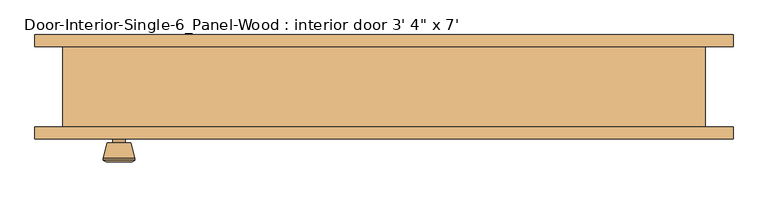
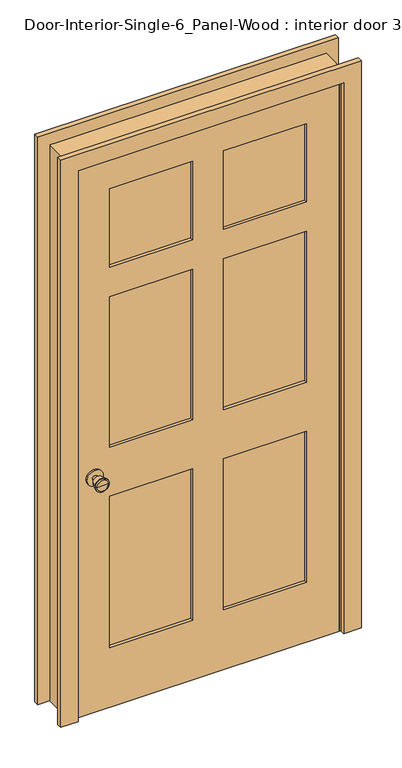
"""IFC4 building model written with IfcOpenShell, lengths in millimetres: door geometry."""

from ifc_helpers import new_model, si_unit, point, frame, frame_2d, origin, place, context, project, spatial, polyline, circle_curve, trimmed, segment, composite_curve, outline, extrude, faceted_brep, source, transform, mapped, element, save
from ifc_brep_helpers import plane_surface, cylinder_surface, revolved_surface, advanced_brep


def door_6a452240(model_context):
    return source(origin(), model_context, "Body", "SolidModel", [
        advanced_brep(
        [(-419.1, -19.4, 914.4), (-429.1, -19.4, 914.4), (-409.1, -19.4, 914.4), (-398.6241324, 29.6, 914.4), (-439.5758676, 29.6, 914.4), (-419.1, 29.6, 914.4), (-394.1, 27.7721319, 914.4), (-444.1, 27.7721319, 914.4), (-394.1, 24.3084537, 914.4), (-444.1, 24.3084537, 914.4), (-400.463764, -0.4, 914.4), (-437.736236, -0.4, 914.4), (-409.1, -0.4, 914.4), (-429.1, -0.4, 914.4)],
        [
            (0, 1),
            (1, 2, circle_curve(frame((-419.1, -19.4, 914.4), z_axis=(0.0, -1.0, 0.0), x_axis=(-1.0, 0.0, 0.0)), 10.0)),
            (2, 0),
            (2, 1, circle_curve(frame((-419.1, -19.4, 914.4), z_axis=(0.0, -1.0, 0.0), x_axis=(-1.0, 0.0, 0.0)), 10.0)),
            (3, 4, circle_curve(frame((-419.1, 29.6, 914.4), z_axis=(0.0, 1.0, 0.0), x_axis=(-1.0, 0.0, 0.0)), 20.4758676)),
            (4, 5),
            (5, 3),
            (4, 3, circle_curve(frame((-419.1, 29.6, 914.4), z_axis=(0.0, 1.0, 0.0), x_axis=(-1.0, 0.0, 0.0)), 20.4758676)),
            (6, 7, circle_curve(frame((-419.1, 27.7721319, 914.4), z_axis=(0.0, 1.0, 0.0), x_axis=(-1.0, 0.0, 0.0)), 25.0)),
            (7, 4),
            (3, 6),
            (7, 6, circle_curve(frame((-419.1, 27.7721319, 914.4), z_axis=(0.0, 1.0, 0.0), x_axis=(-1.0, 0.0, 0.0)), 25.0)),
            (8, 9, circle_curve(frame((-419.1, 24.3084537, 914.4), z_axis=(0.0, 1.0, 0.0), x_axis=(-1.0, 0.0, 0.0)), 25.0)),
            (9, 7),
            (6, 8),
            (9, 8, circle_curve(frame((-419.1, 24.3084537, 914.4), z_axis=(0.0, 1.0, 0.0), x_axis=(-1.0, 0.0, 0.0)), 25.0)),
            (10, 11, circle_curve(frame((-419.1, -0.4, 914.4), z_axis=(0.0, 1.0, 0.0), x_axis=(-1.0, 0.0, 0.0)), 18.636236)),
            (11, 9),
            (8, 10),
            (11, 10, circle_curve(frame((-419.1, -0.4, 914.4), z_axis=(0.0, 1.0, 0.0), x_axis=(-1.0, 0.0, 0.0)), 18.636236)),
            (12, 13, circle_curve(frame((-419.1, -0.4, 914.4), z_axis=(0.0, 1.0, 0.0), x_axis=(-1.0, 0.0, 0.0)), 10.0)),
            (13, 11),
            (10, 12),
            (13, 12, circle_curve(frame((-419.1, -0.4, 914.4), z_axis=(0.0, 1.0, 0.0), x_axis=(-1.0, 0.0, 0.0)), 10.0)),
            (1, 13),
            (12, 2),
        ],
        [
            plane_surface(frame((-419.1, -19.4, 914.4), z_axis=(0.0, -1.0, 0.0), x_axis=(-1.0, 0.0, 0.0))),
            plane_surface(frame((-419.1, 29.6, 914.4), z_axis=(0.0, 1.0, 0.0), x_axis=(-1.0, 0.0, 0.0))),
            revolved_surface(polyline([(-439.5758676, 29.6, 914.4), (-444.1, 27.7721319, 914.4)]), (-419.1, -19.4, 914.4), (0.0, -1.0, 0.0)),
            cylinder_surface(frame((-419.1, -19.4, 914.4), z_axis=(0.0, -1.0, 0.0), x_axis=(-1.0, 0.0, 0.0)), 25.0),
            revolved_surface(polyline([(-444.1, 24.3084537, 914.4), (-437.736236, -0.4, 914.4)]), (-419.1, -19.4, 914.4), (0.0, -1.0, 0.0)),
            plane_surface(frame((-419.1, -0.4, 914.4), z_axis=(0.0, -1.0, 0.0), x_axis=(-1.0, 0.0, 0.0))),
            cylinder_surface(frame((-419.1, -19.4, 914.4), z_axis=(0.0, -1.0, 0.0), x_axis=(-1.0, 0.0, 0.0)), 10.0),
        ],
        [
            (0, [[1, 2, 3]]),
            (0, [[-3, 4, -1]]),
            (1, [[5, 6, 7]]),
            (1, [[8, -7, -6]]),
            (2, [[9, 10, -5, 11]]),
            (2, [[12, -11, -8, -10]]),
            (3, [[13, 14, -9, 15]]),
            (3, [[16, -15, -12, -14]]),
            (4, [[17, 18, -13, 19]]),
            (4, [[20, -19, -16, -18]]),
            (5, [[21, 22, -17, 23]]),
            (5, [[24, -23, -20, -22]]),
            (6, [[-2, 25, -21, 26]]),
            (6, [[-4, -26, -24, -25]]),
        ],
    ),
        extrude(outline(composite_curve([segment(trimmed(circle_curve(frame_2d((914.4, -419.1)), 30.0), [point((914.4, -449.1))], [point((914.4, -389.1))], False, "CARTESIAN"), True, "CONTINUOUS"), segment(trimmed(circle_curve(frame_2d((914.4, -419.1)), 30.0), [point((914.4, -389.1))], [point((914.4, -449.1))], False, "CARTESIAN"), True, "CONTINUOUS")], self_intersect=False)), frame((0.0, -25.4, 0.0), z_axis=(0.0, 1.0, 0.0), x_axis=(0.0, 0.0, 1.0)), (0.0, 0.0, 1.0), 6.0),
        advanced_brep(
        [(-419.1, -66.325, 914.4), (-409.1, -66.325, 914.4), (-429.1, -66.325, 914.4), (-398.6241324, -115.325, 914.4), (-419.1, -115.325, 914.4), (-439.5758676, -115.325, 914.4), (-394.1, -113.4971319, 914.4), (-444.1, -113.4971319, 914.4), (-394.1, -110.0334537, 914.4), (-444.1, -110.0334537, 914.4), (-400.463764, -85.325, 914.4), (-437.736236, -85.325, 914.4), (-409.1, -85.325, 914.4), (-429.1, -85.325, 914.4)],
        [
            (0, 1),
            (1, 2, circle_curve(frame((-419.1, -66.325, 914.4), z_axis=(0.0, 1.0, 0.0), x_axis=(-1.0, 0.0, 0.0)), 10.0)),
            (2, 0),
            (2, 1, circle_curve(frame((-419.1, -66.325, 914.4), z_axis=(0.0, 1.0, 0.0), x_axis=(-1.0, 0.0, 0.0)), 10.0)),
            (3, 4),
            (4, 5),
            (5, 3, circle_curve(frame((-419.1, -115.325, 914.4), z_axis=(0.0, -1.0, 0.0), x_axis=(-1.0, 0.0, 0.0)), 20.4758676)),
            (3, 5, circle_curve(frame((-419.1, -115.325, 914.4), z_axis=(0.0, -1.0, 0.0), x_axis=(-1.0, 0.0, 0.0)), 20.4758676)),
            (6, 3),
            (5, 7),
            (7, 6, circle_curve(frame((-419.1, -113.4971319, 914.4), z_axis=(0.0, -1.0, 0.0), x_axis=(-1.0, 0.0, 0.0)), 25.0)),
            (6, 7, circle_curve(frame((-419.1, -113.4971319, 914.4), z_axis=(0.0, -1.0, 0.0), x_axis=(-1.0, 0.0, 0.0)), 25.0)),
            (8, 6),
            (7, 9),
            (9, 8, circle_curve(frame((-419.1, -110.0334537, 914.4), z_axis=(0.0, -1.0, 0.0), x_axis=(-1.0, 0.0, 0.0)), 25.0)),
            (8, 9, circle_curve(frame((-419.1, -110.0334537, 914.4), z_axis=(0.0, -1.0, 0.0), x_axis=(-1.0, 0.0, 0.0)), 25.0)),
            (10, 8),
            (9, 11),
            (11, 10, circle_curve(frame((-419.1, -85.325, 914.4), z_axis=(0.0, -1.0, 0.0), x_axis=(-1.0, 0.0, 0.0)), 18.636236)),
            (10, 11, circle_curve(frame((-419.1, -85.325, 914.4), z_axis=(0.0, -1.0, 0.0), x_axis=(-1.0, 0.0, 0.0)), 18.636236)),
            (12, 10),
            (11, 13),
            (13, 12, circle_curve(frame((-419.1, -85.325, 914.4), z_axis=(0.0, -1.0, 0.0), x_axis=(-1.0, 0.0, 0.0)), 10.0)),
            (12, 13, circle_curve(frame((-419.1, -85.325, 914.4), z_axis=(0.0, -1.0, 0.0), x_axis=(-1.0, 0.0, 0.0)), 10.0)),
            (1, 12),
            (13, 2),
        ],
        [
            plane_surface(frame((-419.1, -66.325, 914.4), z_axis=(0.0, 1.0, 0.0), x_axis=(-1.0, 0.0, 0.0))),
            plane_surface(frame((-419.1, -115.325, 914.4), z_axis=(0.0, -1.0, 0.0), x_axis=(-1.0, 0.0, 0.0))),
            revolved_surface(polyline([(-439.5758676, -115.325, 914.4), (-444.1, -113.4971319, 914.4)]), (-419.1, -66.325, 914.4), (0.0, 1.0, 0.0)),
            cylinder_surface(frame((-419.1, -66.325, 914.4), z_axis=(0.0, 1.0, 0.0), x_axis=(-1.0, 0.0, 0.0)), 25.0),
            revolved_surface(polyline([(-444.1, -110.0334537, 914.4), (-437.736236, -85.325, 914.4)]), (-419.1, -66.325, 914.4), (0.0, 1.0, 0.0)),
            plane_surface(frame((-419.1, -85.325, 914.4), z_axis=(0.0, 1.0, 0.0), x_axis=(-1.0, 0.0, 0.0))),
            cylinder_surface(frame((-419.1, -66.325, 914.4), z_axis=(0.0, 1.0, 0.0), x_axis=(-1.0, 0.0, 0.0)), 10.0),
        ],
        [
            (0, [[1, 2, 3]]),
            (0, [[-3, 4, -1]]),
            (1, [[5, 6, 7]]),
            (1, [[-6, -5, 8]]),
            (2, [[9, -7, 10, 11]]),
            (2, [[-10, -8, -9, 12]]),
            (3, [[13, -11, 14, 15]]),
            (3, [[-14, -12, -13, 16]]),
            (4, [[17, -15, 18, 19]]),
            (4, [[-18, -16, -17, 20]]),
            (5, [[21, -19, 22, 23]]),
            (5, [[-22, -20, -21, 24]]),
            (6, [[25, -23, 26, -2]]),
            (6, [[-26, -24, -25, -4]]),
        ],
    ),
        extrude(outline(composite_curve([segment(trimmed(circle_curve(frame_2d((914.4, -419.1)), 30.0), [point((914.4, -449.1))], [point((914.4, -389.1))], False, "CARTESIAN"), True, "CONTINUOUS"), segment(trimmed(circle_curve(frame_2d((914.4, -419.1)), 30.0), [point((914.4, -389.1))], [point((914.4, -449.1))], False, "CARTESIAN"), True, "CONTINUOUS")], self_intersect=False)), frame((0.0, -66.325, 0.0), z_axis=(0.0, 1.0, 0.0), x_axis=(0.0, 0.0, 1.0)), (0.0, 0.0, 1.0), 6.0),
        faceted_brep([(508.0, -60.325, 0.0), (482.6, -60.325, 0.0), (482.6, -25.4, 0.0), (469.9, -25.4, 0.0), (469.9, 9.525, 0.0), (482.6, 9.525, 0.0), (482.6, 66.675, 0.0), (508.0, 66.675, 0.0), (508.0, 66.675, 2159.0), (508.0, -60.325, 2159.0), (482.6, 66.675, 2133.6), (-482.6, 66.675, 2133.6), (-482.6, 66.675, 0.0), (-508.0, 66.675, 0.0), (-508.0, 66.675, 2159.0), (482.6, 9.525, 2133.6), (469.9, 9.525, 2120.9), (-469.9, 9.525, 2120.9), (-469.9, 9.525, 0.0), (-482.6, 9.525, 0.0), (-482.6, 9.525, 2133.6), (469.9, -25.4, 2120.9), (482.6, -25.4, 2133.6), (-482.6, -25.4, 2133.6), (-482.6, -25.4, 0.0), (-469.9, -25.4, 0.0), (-469.9, -25.4, 2120.9), (482.6, -60.325, 2133.6), (-508.0, -60.325, 2159.0), (-508.0, -60.325, 0.0), (-482.6, -60.325, 0.0), (-482.6, -60.325, 2133.6)], [[[0, 1, 2, 3, 4, 5, 6, 7]], [[7, 8, 9, 0]], [[6, 10, 11, 12, 13, 14, 8, 7]], [[5, 15, 10, 6]], [[4, 16, 17, 18, 19, 20, 15, 5]], [[3, 21, 16, 4]], [[2, 22, 23, 24, 25, 26, 21, 3]], [[1, 27, 22, 2]], [[0, 9, 28, 29, 30, 31, 27, 1]], [[8, 14, 28, 9]], [[15, 20, 11, 10]], [[21, 26, 17, 16]], [[27, 31, 23, 22]], [[29, 13, 12, 19, 18, 25, 24, 30]], [[14, 13, 29, 28]], [[20, 19, 12, 11]], [[26, 25, 18, 17]], [[31, 30, 24, 23]]]),
        extrude(outline(polyline([(2133.6, -482.6), (0.0, -482.6), (0.0, 482.6), (2133.6, 482.6), (2133.6, -482.6)]), holes=[polyline([(2014.5375, 57.15), (2014.5375, 361.95), (1709.7375, 361.95), (1709.7375, 57.15), (2014.5375, 57.15)]), polyline([(1595.4375, 361.95), (1009.65, 361.95), (1009.65, 57.15), (1595.4375, 57.15), (1595.4375, 361.95)]), polyline([(1009.65, -57.15), (1009.65, -361.95), (1595.4375, -361.95), (1595.4375, -57.15), (1009.65, -57.15)]), polyline([(1709.7375, -361.95), (2014.5375, -361.95), (2014.5375, -57.15), (1709.7375, -57.15), (1709.7375, -361.95)]), polyline([(819.15, 57.15), (819.15, 361.95), (231.775, 361.95), (231.775, 57.15), (819.15, 57.15)]), polyline([(231.775, -57.15), (231.775, -361.95), (819.15, -361.95), (819.15, -57.15), (231.775, -57.15)])]), frame((0.0, -60.325, 0.0), z_axis=(0.0, 1.0, 0.0), x_axis=(0.0, 0.0, 1.0)), (0.0, 0.0, 1.0), 34.925),
        extrude(outline(polyline([(361.95, -37.0416667), (361.95, -48.6833333), (57.15, -48.6833333), (57.15, -37.0416667), (361.95, -37.0416667)])), frame((0.0, 0.0, 1709.7375), z_axis=(0.0, 0.0, 1.0), x_axis=(1.0, 0.0, 0.0)), (0.0, 0.0, 1.0), 304.8),
        extrude(outline(polyline([(361.95, -37.0416667), (361.95, -48.6833333), (57.15, -48.6833333), (57.15, -37.0416667), (361.95, -37.0416667)])), frame((0.0, 0.0, 1009.65), z_axis=(0.0, 0.0, 1.0), x_axis=(1.0, 0.0, 0.0)), (0.0, 0.0, 1.0), 585.7875),
        extrude(outline(polyline([(-57.15, -37.0416667), (-57.15, -48.6833333), (-361.95, -48.6833333), (-361.95, -37.0416667), (-57.15, -37.0416667)])), frame((0.0, 0.0, 1009.65), z_axis=(0.0, 0.0, 1.0), x_axis=(1.0, 0.0, 0.0)), (0.0, 0.0, 1.0), 585.7875),
        extrude(outline(polyline([(-57.15, -37.0416667), (-57.15, -48.6833333), (-361.95, -48.6833333), (-361.95, -37.0416667), (-57.15, -37.0416667)])), frame((0.0, 0.0, 1709.7375), z_axis=(0.0, 0.0, 1.0), x_axis=(1.0, 0.0, 0.0)), (0.0, 0.0, 1.0), 304.8),
        extrude(outline(polyline([(361.95, -37.0416667), (361.95, -48.6833333), (57.15, -48.6833333), (57.15, -37.0416667), (361.95, -37.0416667)])), frame((0.0, 0.0, 231.775), z_axis=(0.0, 0.0, 1.0), x_axis=(1.0, 0.0, 0.0)), (0.0, 0.0, 1.0), 587.375),
        extrude(outline(polyline([(-57.15, -37.0416667), (-57.15, -48.6833333), (-361.95, -48.6833333), (-361.95, -37.0416667), (-57.15, -37.0416667)])), frame((0.0, 0.0, 231.775), z_axis=(0.0, 0.0, 1.0), x_axis=(1.0, 0.0, 0.0)), (0.0, 0.0, 1.0), 587.375),
        extrude(outline(polyline([(0.0, 552.45), (2203.45, 552.45), (2203.45, -552.45), (0.0, -552.45), (0.0, -488.95), (2139.95, -488.95), (2139.95, 488.95), (0.0, 488.95), (0.0, 552.45)])), frame((0.0, -79.375, 0.0), z_axis=(0.0, 1.0, 0.0), x_axis=(0.0, 0.0, 1.0)), (0.0, 0.0, 1.0), 19.05),
        extrude(outline(polyline([(0.0, 552.45), (2203.45, 552.45), (2203.45, -552.45), (0.0, -552.45), (0.0, -488.95), (2139.95, -488.95), (2139.95, 488.95), (0.0, 488.95), (0.0, 552.45)])), frame((0.0, 66.675, 0.0), z_axis=(0.0, 1.0, 0.0), x_axis=(0.0, 0.0, 1.0)), (0.0, 0.0, 1.0), 19.05),
    ])


if __name__ == "__main__":
    model = new_model("IFC4")
    model_context = context("Model", 3, world=origin())
    ifc_project = project(units=[si_unit("LENGTHUNIT", "METRE", prefix="MILLI")], contexts=[model_context])
    site = spatial("IfcSite", under=ifc_project)
    building = spatial("IfcBuilding", under=site)
    placement = place(None, origin())
    door_shape = door_6a452240(model_context)
    element("IfcDoor", 1, ObjectType="Door-Interior-Single-6_Panel-Wood : interior door 3' 4\" x 7'", at=placement, inside=building, context=model_context, shape_type="MappedRepresentation", body=[
        mapped(door_shape, transform((0.0, 0.0, 0.0), x_axis=(1.0, 0.0, 0.0), y_axis=(0.0, 1.0, 0.0), z_axis=(0.0, 0.0, 1.0))),
    ])
    save(model, "model.ifc")

# Revit data of these elements
# Type "Door-Interior-Single-6_Panel-Wood : interior door 3' 4\" x 7'"
#   Type Mark = "11"
#   Assembly Code = "C1020300"
#   Analytic Construction = "Wooden"
#   Top Rail = 0' - 4 11/16"
#   Top Panel = 1' - 0"
#   Thickness = 0' - 1 3/8"
#   Thermal Resistance (R) = 2.5876 (h·ft²·°F)/BTU
#   Swing Angle [instance default] = 90.00°
#   Stiles = 0' - 4 3/4"
#   Rough Width = 3' - 4"
#   Rough Height = 7' - 1"
#   Mullion = 0' - 4 1/2"
#   Lock Rail = 0' - 7 1/2"
#   Intermediate Rail = 0' - 4 1/2"
#   Height = 7' - 0"
#   Width = 3' - 2"
#   Heat Transfer Coefficient (U) = 0.3865 BTU/(h·ft²·°F)
#   Bottom Rail = 0' - 9 1/8"
#   Trim Material = Cherry
#   Panel Material = Cherry
#   Frame Material = Cherry
#   Door Handle Material = Aluminum
#   Visual Light Transmittance = 0
#   Solar Heat Gain Coefficient = 0
#   Wall Closure = (empty or 0)
#   Function = (empty or 0)
# Element 1 (IfcDoor, "Door-Interior-Single-6_Panel-Wood : interior door 3' 4\" x 7'")
#   Materials on its faces: "Cherry", "Aluminum"
# Materials
#   "Cherry": class "Wood", colour RGB 226 177 128, transparency 0, Description = "Prunus Serotina", Cost = 0
#   "Aluminum": class "Metal", colour RGB 247 247 247, transparency 0, Description = "Aluminum 6061", Cost = 0
